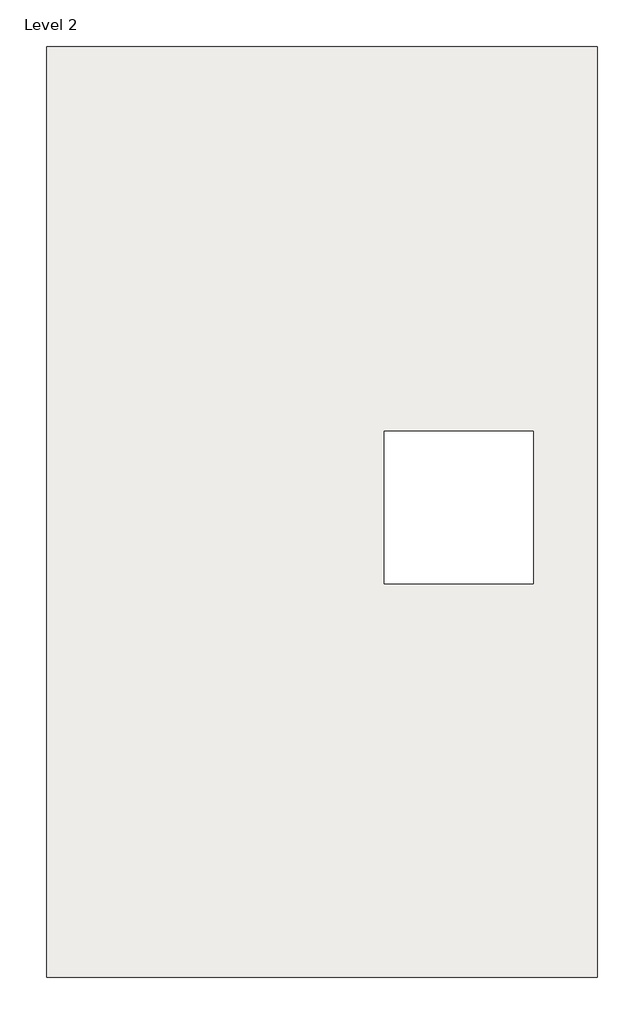
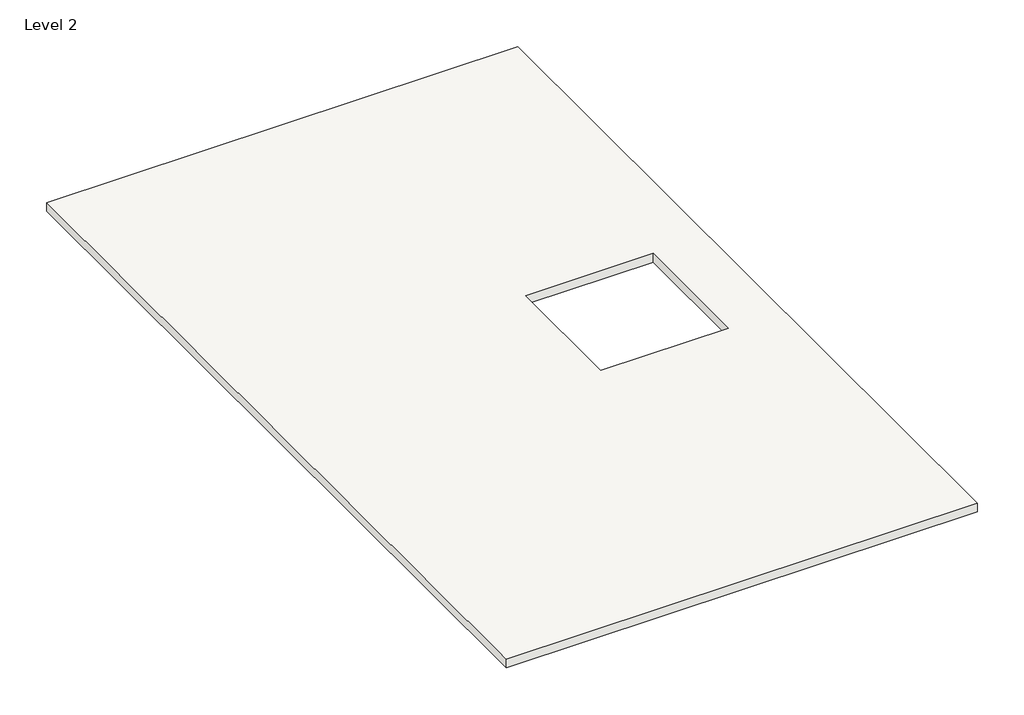
# One storey, incomplete: 1 roof.
"""IFC4 building model written with IfcOpenShell, lengths in millimetres."""

from ifc_helpers import new_model, si_unit, frame, origin, place, context, project, spatial, polyline, outline, extrude, element, save

model = new_model("IFC4")

# Units and contexts
model_context = context("Model", 3, world=origin())
ifc_project = project(units=[si_unit("LENGTHUNIT", "METRE", prefix="MILLI")], contexts=[model_context])

# Site, building, storey
site = spatial("IfcSite", under=ifc_project)
building = spatial("IfcBuilding", under=site)
storey = spatial("IfcBuildingStorey", under=building, Name="Level 2", Elevation=3048.0)

# Roof
placement = place(None, origin())
element("IfcRoof", 1, ObjectType="ROOF 6\"", at=placement, inside=storey, context=model_context, shape_type="SweptSolid", body=[
    extrude(outline(polyline([(-5720.6138307, -6924.1482799), (-5720.6138307, 6410.8517201), (2166.0861693, 6410.8517201), (2166.0861693, -6924.1482799), (-5720.6138307, -6924.1482799)]), holes=[polyline([(1251.6861693, -1285.3482799), (1251.6861693, 899.0517201), (-881.9138307, 899.0517201), (-881.9138307, -1285.3482799), (1251.6861693, -1285.3482799)])]), frame((0.0, 0.0, 3048.0), z_axis=(0.0, 0.0, 1.0), x_axis=(1.0, 0.0, 0.0)), (0.0, 0.0, 1.0), 152.4),
])

save(model, "model.ifc")

# Revit data of these elements
# Type "ROOF 6\""
#   Assembly Code = "B1020"
#   Layers, outside or top first: 0' - 6" no material (function 1)
# Element 1 (IfcRoof, "ROOF 6\"")
#   built-in parameter 1001705 = 10.5 (stored number, unit not read)
#   built-in parameter 1001710 = 33615
#   Phase Created = New Construction
#   Materials on its faces: "Default Roof", "Door - Panel"
# Materials
#   "Default Roof": colour RGB 88 101 114, transparency 0, Cost = 0
#   "Door - Panel": class "Wood", colour RGB 210 159 95, transparency 0, Cost = 0
